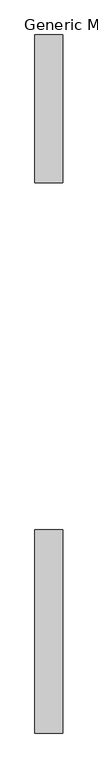
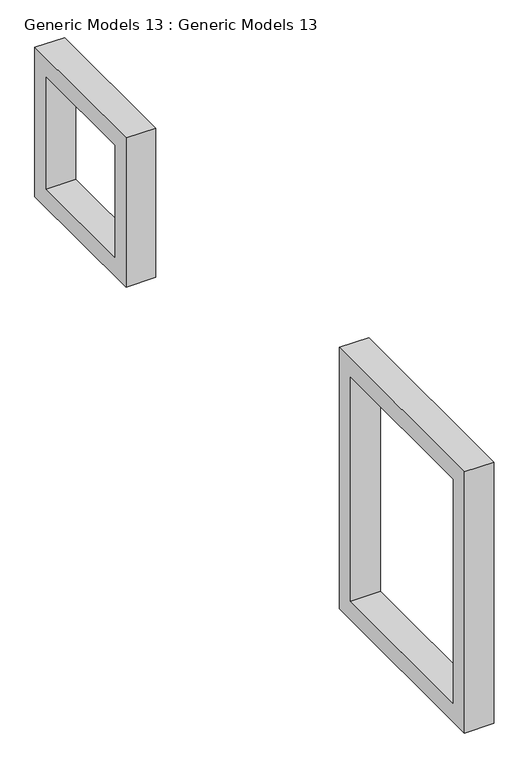
"""IFC4 building model written with IfcOpenShell, lengths in millimetres: proxy geometry, Generic Models 13 : Generic Models 13."""

from ifc_helpers import new_model, si_unit, frame, origin, place, context, project, spatial, polyline, outline, extrude, source, transform, mapped, element, save


def generic_models_13_generic_models_13_70bfc34e(model_context):
    return source(origin(), model_context, "Body", "SweptSolid", [
        extrude(outline(polyline([(7048.5641252, 3243.5849297), (7861.3641252, 3243.5849297), (7861.3641252, 2430.7849297), (7048.5641252, 2430.7849297), (7048.5641252, 3243.5849297)]), holes=[polyline([(7150.1641252, 3141.9849297), (7150.1641252, 2532.3849297), (7759.7641252, 2532.3849297), (7759.7641252, 3141.9849297), (7150.1641252, 3141.9849297)])]), frame((-6249.8280307, 0.0, 0.0), z_axis=(1.0, 0.0, 0.0), x_axis=(0.0, 1.0, 0.0)), (0.0, 0.0, 1.0), 152.4),
        extrude(outline(polyline([(4025.9641252, 3257.8433359), (5143.5641252, 3257.8433359), (5143.5641252, 1835.4433359), (4025.9641252, 1835.4433359), (4025.9641252, 3257.8433359)]), holes=[polyline([(4127.5641252, 3156.2433359), (4127.5641252, 1937.0433359), (5041.9641252, 1937.0433359), (5041.9641252, 3156.2433359), (4127.5641252, 3156.2433359)])]), frame((-6249.8280307, 0.0, 0.0), z_axis=(1.0, 0.0, 0.0), x_axis=(0.0, 1.0, 0.0)), (0.0, 0.0, 1.0), 152.4),
    ])


if __name__ == "__main__":
    model = new_model("IFC4")
    model_context = context("Model", 3, world=origin())
    ifc_project = project(units=[si_unit("LENGTHUNIT", "METRE", prefix="MILLI")], contexts=[model_context])
    site = spatial("IfcSite", under=ifc_project)
    building = spatial("IfcBuilding", under=site)
    placement = place(None, origin())
    generic_models_13_generic_models_13_shape = generic_models_13_generic_models_13_70bfc34e(model_context)
    element("IfcBuildingElementProxy", 1, Name="Generic Models 13 : Generic Models 13", ObjectType="Generic Models 13 : Generic Models 13", at=placement, inside=building, context=model_context, shape_type="MappedRepresentation", body=[
        mapped(generic_models_13_generic_models_13_shape, transform((0.0, 0.0, 0.0), x_axis=(1.0, 0.0, 0.0), y_axis=(0.0, 1.0, 0.0), z_axis=(0.0, 0.0, 1.0))),
    ])
    save(model, "model.ifc")

# Revit data of these elements
# Element 1 (IfcBuildingElementProxy, "Generic Models 13 : Generic Models 13")
#   Materials on its faces: "chocolate brown"
# Materials
#   "chocolate brown": class "Generic", colour RGB 120 120 120, transparency 0, Cost = 0
